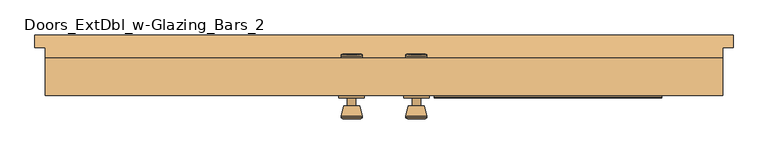
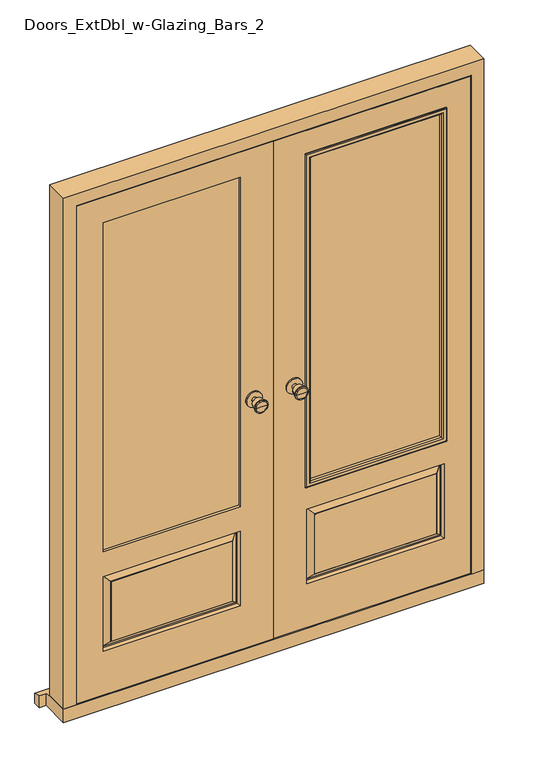
"""IFC4 building model written with IfcOpenShell, lengths in millimetres: door geometry, Doors_ExtDbl_w-Glazing_Bars_2."""

from ifc_helpers import new_model, si_unit, point, frame, frame_2d, origin, place, context, project, spatial, polyline, circle_curve, ellipse_curve, trimmed, segment, composite_curve, outline, extrude, faceted_brep, source, transform, mapped, element, save
from ifc_brep_helpers import plane_surface, cylinder_surface, revolved_surface, advanced_brep


def doors_extdbl_w_glazing_bars_2_f0b4ebcb(model_context):
    return source(origin(), model_context, "Body", "SolidModel", [
        advanced_brep(
        [(76.5, -5.7, 1050.0), (86.5, -5.7, 1050.0), (66.5, -5.7, 1050.0), (96.9758676, -54.7, 1050.0), (76.5, -54.7, 1050.0), (56.0241324, -54.7, 1050.0), (101.5, -52.8721319, 1050.0), (51.5, -52.8721319, 1050.0), (101.5, -49.4084537, 1050.0), (51.5, -49.4084537, 1050.0), (95.136236, -24.7, 1050.0), (57.863764, -24.7, 1050.0), (86.5, -24.7, 1050.0), (66.5, -24.7, 1050.0)],
        [
            (0, 1),
            (1, 2, circle_curve(frame((76.5, -5.7, 1050.0), z_axis=(0.0, 1.0, 0.0), x_axis=(-1.0, 0.0, 0.0)), 10.0)),
            (2, 0),
            (2, 1, circle_curve(frame((76.5, -5.7, 1050.0), z_axis=(0.0, 1.0, 0.0), x_axis=(-1.0, 0.0, 0.0)), 10.0)),
            (3, 4),
            (4, 5),
            (5, 3, circle_curve(frame((76.5, -54.7, 1050.0), z_axis=(0.0, -1.0, 0.0), x_axis=(-1.0, 0.0, 0.0)), 20.4758676)),
            (3, 5, circle_curve(frame((76.5, -54.7, 1050.0), z_axis=(0.0, -1.0, 0.0), x_axis=(-1.0, 0.0, 0.0)), 20.4758676)),
            (6, 3),
            (5, 7),
            (7, 6, circle_curve(frame((76.5, -52.8721319, 1050.0), z_axis=(0.0, -1.0, 0.0), x_axis=(-1.0, 0.0, 0.0)), 25.0)),
            (6, 7, circle_curve(frame((76.5, -52.8721319, 1050.0), z_axis=(0.0, -1.0, 0.0), x_axis=(-1.0, 0.0, 0.0)), 25.0)),
            (8, 6),
            (7, 9),
            (9, 8, circle_curve(frame((76.5, -49.4084537, 1050.0), z_axis=(0.0, -1.0, 0.0), x_axis=(-1.0, 0.0, 0.0)), 25.0)),
            (8, 9, circle_curve(frame((76.5, -49.4084537, 1050.0), z_axis=(0.0, -1.0, 0.0), x_axis=(-1.0, 0.0, 0.0)), 25.0)),
            (10, 8),
            (9, 11),
            (11, 10, circle_curve(frame((76.5, -24.7, 1050.0), z_axis=(0.0, -1.0, 0.0), x_axis=(-1.0, 0.0, 0.0)), 18.636236)),
            (10, 11, circle_curve(frame((76.5, -24.7, 1050.0), z_axis=(0.0, -1.0, 0.0), x_axis=(-1.0, 0.0, 0.0)), 18.636236)),
            (12, 10),
            (11, 13),
            (13, 12, circle_curve(frame((76.5, -24.7, 1050.0), z_axis=(0.0, -1.0, 0.0), x_axis=(-1.0, 0.0, 0.0)), 10.0)),
            (12, 13, circle_curve(frame((76.5, -24.7, 1050.0), z_axis=(0.0, -1.0, 0.0), x_axis=(-1.0, 0.0, 0.0)), 10.0)),
            (1, 12),
            (13, 2),
        ],
        [
            plane_surface(frame((76.5, -5.7, 1050.0), z_axis=(0.0, 1.0, 0.0), x_axis=(-1.0, 0.0, 0.0))),
            plane_surface(frame((76.5, -54.7, 1050.0), z_axis=(0.0, -1.0, 0.0), x_axis=(-1.0, 0.0, 0.0))),
            revolved_surface(polyline([(56.0241324, -54.7, 1050.0), (51.5, -52.8721319, 1050.0)]), (76.5, -5.7, 1050.0), (0.0, 1.0, 0.0)),
            cylinder_surface(frame((76.5, -5.7, 1050.0), z_axis=(0.0, 1.0, 0.0), x_axis=(-1.0, 0.0, 0.0)), 25.0),
            revolved_surface(polyline([(51.5, -49.4084537, 1050.0), (57.863764, -24.7, 1050.0)]), (76.5, -5.7, 1050.0), (0.0, 1.0, 0.0)),
            plane_surface(frame((76.5, -24.7, 1050.0), z_axis=(0.0, 1.0, 0.0), x_axis=(-1.0, 0.0, 0.0))),
            cylinder_surface(frame((76.5, -5.7, 1050.0), z_axis=(0.0, 1.0, 0.0), x_axis=(-1.0, 0.0, 0.0)), 10.0),
        ],
        [
            (0, [[1, 2, 3]]),
            (0, [[-3, 4, -1]]),
            (1, [[5, 6, 7]]),
            (1, [[-6, -5, 8]]),
            (2, [[9, -7, 10, 11]]),
            (2, [[-10, -8, -9, 12]]),
            (3, [[13, -11, 14, 15]]),
            (3, [[-14, -12, -13, 16]]),
            (4, [[17, -15, 18, 19]]),
            (4, [[-18, -16, -17, 20]]),
            (5, [[21, -19, 22, 23]]),
            (5, [[-22, -20, -21, 24]]),
            (6, [[25, -23, 26, -2]]),
            (6, [[-26, -24, -25, -4]]),
        ],
    ),
        extrude(outline(composite_curve([segment(trimmed(circle_curve(frame_2d((1050.0, 76.5)), 30.0), [point((1050.0, 46.5))], [point((1050.0, 106.5))], False, "CARTESIAN"), True, "CONTINUOUS"), segment(trimmed(circle_curve(frame_2d((1050.0, 76.5)), 30.0), [point((1050.0, 106.5))], [point((1050.0, 46.5))], False, "CARTESIAN"), True, "CONTINUOUS")], self_intersect=False)), frame((0.0, -5.7, 0.0), z_axis=(0.0, 1.0, 0.0), x_axis=(0.0, 0.0, 1.0)), (0.0, 0.0, 1.0), 6.0),
        advanced_brep(
        [(76.5, 50.3, 1050.0), (66.5, 50.3, 1050.0), (86.5, 50.3, 1050.0), (96.9758676, 99.3, 1050.0), (56.0241324, 99.3, 1050.0), (76.5, 99.3, 1050.0), (101.5, 97.4721319, 1050.0), (51.5, 97.4721319, 1050.0), (101.5, 94.0084537, 1050.0), (51.5, 94.0084537, 1050.0), (95.136236, 69.3, 1050.0), (57.863764, 69.3, 1050.0), (86.5, 69.3, 1050.0), (66.5, 69.3, 1050.0)],
        [
            (0, 1),
            (1, 2, circle_curve(frame((76.5, 50.3, 1050.0), z_axis=(0.0, -1.0, 0.0), x_axis=(-1.0, 0.0, 0.0)), 10.0)),
            (2, 0),
            (2, 1, circle_curve(frame((76.5, 50.3, 1050.0), z_axis=(0.0, -1.0, 0.0), x_axis=(-1.0, 0.0, 0.0)), 10.0)),
            (3, 4, circle_curve(frame((76.5, 99.3, 1050.0), z_axis=(0.0, 1.0, 0.0), x_axis=(-1.0, 0.0, 0.0)), 20.4758676)),
            (4, 5),
            (5, 3),
            (4, 3, circle_curve(frame((76.5, 99.3, 1050.0), z_axis=(0.0, 1.0, 0.0), x_axis=(-1.0, 0.0, 0.0)), 20.4758676)),
            (6, 7, circle_curve(frame((76.5, 97.4721319, 1050.0), z_axis=(0.0, 1.0, 0.0), x_axis=(-1.0, 0.0, 0.0)), 25.0)),
            (7, 4),
            (3, 6),
            (7, 6, circle_curve(frame((76.5, 97.4721319, 1050.0), z_axis=(0.0, 1.0, 0.0), x_axis=(-1.0, 0.0, 0.0)), 25.0)),
            (8, 9, circle_curve(frame((76.5, 94.0084537, 1050.0), z_axis=(0.0, 1.0, 0.0), x_axis=(-1.0, 0.0, 0.0)), 25.0)),
            (9, 7),
            (6, 8),
            (9, 8, circle_curve(frame((76.5, 94.0084537, 1050.0), z_axis=(0.0, 1.0, 0.0), x_axis=(-1.0, 0.0, 0.0)), 25.0)),
            (10, 11, circle_curve(frame((76.5, 69.3, 1050.0), z_axis=(0.0, 1.0, 0.0), x_axis=(-1.0, 0.0, 0.0)), 18.636236)),
            (11, 9),
            (8, 10),
            (11, 10, circle_curve(frame((76.5, 69.3, 1050.0), z_axis=(0.0, 1.0, 0.0), x_axis=(-1.0, 0.0, 0.0)), 18.636236)),
            (12, 13, circle_curve(frame((76.5, 69.3, 1050.0), z_axis=(0.0, 1.0, 0.0), x_axis=(-1.0, 0.0, 0.0)), 10.0)),
            (13, 11),
            (10, 12),
            (13, 12, circle_curve(frame((76.5, 69.3, 1050.0), z_axis=(0.0, 1.0, 0.0), x_axis=(-1.0, 0.0, 0.0)), 10.0)),
            (1, 13),
            (12, 2),
        ],
        [
            plane_surface(frame((76.5, 50.3, 1050.0), z_axis=(0.0, -1.0, 0.0), x_axis=(-1.0, 0.0, 0.0))),
            plane_surface(frame((76.5, 99.3, 1050.0), z_axis=(0.0, 1.0, 0.0), x_axis=(-1.0, 0.0, 0.0))),
            revolved_surface(polyline([(56.0241324, 99.3, 1050.0), (51.5, 97.4721319, 1050.0)]), (76.5, 50.3, 1050.0), (0.0, -1.0, 0.0)),
            cylinder_surface(frame((76.5, 50.3, 1050.0), z_axis=(0.0, -1.0, 0.0), x_axis=(-1.0, 0.0, 0.0)), 25.0),
            revolved_surface(polyline([(51.5, 94.0084537, 1050.0), (57.863764, 69.3, 1050.0)]), (76.5, 50.3, 1050.0), (0.0, -1.0, 0.0)),
            plane_surface(frame((76.5, 69.3, 1050.0), z_axis=(0.0, -1.0, 0.0), x_axis=(-1.0, 0.0, 0.0))),
            cylinder_surface(frame((76.5, 50.3, 1050.0), z_axis=(0.0, -1.0, 0.0), x_axis=(-1.0, 0.0, 0.0)), 10.0),
        ],
        [
            (0, [[1, 2, 3]]),
            (0, [[-3, 4, -1]]),
            (1, [[5, 6, 7]]),
            (1, [[8, -7, -6]]),
            (2, [[9, 10, -5, 11]]),
            (2, [[12, -11, -8, -10]]),
            (3, [[13, 14, -9, 15]]),
            (3, [[16, -15, -12, -14]]),
            (4, [[17, 18, -13, 19]]),
            (4, [[20, -19, -16, -18]]),
            (5, [[21, 22, -17, 23]]),
            (5, [[24, -23, -20, -22]]),
            (6, [[-2, 25, -21, 26]]),
            (6, [[-4, -26, -24, -25]]),
        ],
    ),
        extrude(outline(composite_curve([segment(trimmed(circle_curve(frame_2d((1050.0, 76.5)), 30.0), [point((1050.0, 46.5))], [point((1050.0, 106.5))], False, "CARTESIAN"), True, "CONTINUOUS"), segment(trimmed(circle_curve(frame_2d((1050.0, 76.5)), 30.0), [point((1050.0, 106.5))], [point((1050.0, 46.5))], False, "CARTESIAN"), True, "CONTINUOUS")], self_intersect=False)), frame((0.0, 44.3, 0.0), z_axis=(0.0, 1.0, 0.0), x_axis=(0.0, 0.0, 1.0)), (0.0, 0.0, 1.0), 6.0),
        advanced_brep(
        [(-76.5, -5.7, 1050.0), (-66.5, -5.7, 1050.0), (-86.5, -5.7, 1050.0), (-56.0241324, -54.7, 1050.0), (-76.5, -54.7, 1050.0), (-96.9758676, -54.7, 1050.0), (-51.5, -52.8721319, 1050.0), (-101.5, -52.8721319, 1050.0), (-51.5, -49.4084537, 1050.0), (-101.5, -49.4084537, 1050.0), (-57.863764, -24.7, 1050.0), (-95.136236, -24.7, 1050.0), (-66.5, -24.7, 1050.0), (-86.5, -24.7, 1050.0)],
        [
            (0, 1),
            (1, 2, circle_curve(frame((-76.5, -5.7, 1050.0), z_axis=(0.0, 1.0, 0.0), x_axis=(-1.0, 0.0, 0.0)), 10.0)),
            (2, 0),
            (2, 1, circle_curve(frame((-76.5, -5.7, 1050.0), z_axis=(0.0, 1.0, 0.0), x_axis=(-1.0, 0.0, 0.0)), 10.0)),
            (3, 4),
            (4, 5),
            (5, 3, circle_curve(frame((-76.5, -54.7, 1050.0), z_axis=(0.0, -1.0, 0.0), x_axis=(-1.0, 0.0, 0.0)), 20.4758676)),
            (3, 5, circle_curve(frame((-76.5, -54.7, 1050.0), z_axis=(0.0, -1.0, 0.0), x_axis=(-1.0, 0.0, 0.0)), 20.4758676)),
            (6, 3),
            (5, 7),
            (7, 6, circle_curve(frame((-76.5, -52.8721319, 1050.0), z_axis=(0.0, -1.0, 0.0), x_axis=(-1.0, 0.0, 0.0)), 25.0)),
            (6, 7, circle_curve(frame((-76.5, -52.8721319, 1050.0), z_axis=(0.0, -1.0, 0.0), x_axis=(-1.0, 0.0, 0.0)), 25.0)),
            (8, 6),
            (7, 9),
            (9, 8, circle_curve(frame((-76.5, -49.4084537, 1050.0), z_axis=(0.0, -1.0, 0.0), x_axis=(-1.0, 0.0, 0.0)), 25.0)),
            (8, 9, circle_curve(frame((-76.5, -49.4084537, 1050.0), z_axis=(0.0, -1.0, 0.0), x_axis=(-1.0, 0.0, 0.0)), 25.0)),
            (10, 8),
            (9, 11),
            (11, 10, circle_curve(frame((-76.5, -24.7, 1050.0), z_axis=(0.0, -1.0, 0.0), x_axis=(-1.0, 0.0, 0.0)), 18.636236)),
            (10, 11, circle_curve(frame((-76.5, -24.7, 1050.0), z_axis=(0.0, -1.0, 0.0), x_axis=(-1.0, 0.0, 0.0)), 18.636236)),
            (12, 10),
            (11, 13),
            (13, 12, circle_curve(frame((-76.5, -24.7, 1050.0), z_axis=(0.0, -1.0, 0.0), x_axis=(-1.0, 0.0, 0.0)), 10.0)),
            (12, 13, circle_curve(frame((-76.5, -24.7, 1050.0), z_axis=(0.0, -1.0, 0.0), x_axis=(-1.0, 0.0, 0.0)), 10.0)),
            (1, 12),
            (13, 2),
        ],
        [
            plane_surface(frame((-76.5, -5.7, 1050.0), z_axis=(0.0, 1.0, 0.0), x_axis=(-1.0, 0.0, 0.0))),
            plane_surface(frame((-76.5, -54.7, 1050.0), z_axis=(0.0, -1.0, 0.0), x_axis=(-1.0, 0.0, 0.0))),
            revolved_surface(polyline([(-96.9758676, -54.7, 1050.0), (-101.5, -52.8721319, 1050.0)]), (-76.5, -5.7, 1050.0), (0.0, 1.0, 0.0)),
            cylinder_surface(frame((-76.5, -5.7, 1050.0), z_axis=(0.0, 1.0, 0.0), x_axis=(-1.0, 0.0, 0.0)), 25.0),
            revolved_surface(polyline([(-101.5, -49.4084537, 1050.0), (-95.136236, -24.7, 1050.0)]), (-76.5, -5.7, 1050.0), (0.0, 1.0, 0.0)),
            plane_surface(frame((-76.5, -24.7, 1050.0), z_axis=(0.0, 1.0, 0.0), x_axis=(-1.0, 0.0, 0.0))),
            cylinder_surface(frame((-76.5, -5.7, 1050.0), z_axis=(0.0, 1.0, 0.0), x_axis=(-1.0, 0.0, 0.0)), 10.0),
        ],
        [
            (0, [[1, 2, 3]]),
            (0, [[-3, 4, -1]]),
            (1, [[5, 6, 7]]),
            (1, [[-6, -5, 8]]),
            (2, [[9, -7, 10, 11]]),
            (2, [[-10, -8, -9, 12]]),
            (3, [[13, -11, 14, 15]]),
            (3, [[-14, -12, -13, 16]]),
            (4, [[17, -15, 18, 19]]),
            (4, [[-18, -16, -17, 20]]),
            (5, [[21, -19, 22, 23]]),
            (5, [[-22, -20, -21, 24]]),
            (6, [[25, -23, 26, -2]]),
            (6, [[-26, -24, -25, -4]]),
        ],
    ),
        extrude(outline(composite_curve([segment(trimmed(circle_curve(frame_2d((1050.0, -76.5)), 30.0), [point((1050.0, -106.5))], [point((1050.0, -46.5))], False, "CARTESIAN"), True, "CONTINUOUS"), segment(trimmed(circle_curve(frame_2d((1050.0, -76.5)), 30.0), [point((1050.0, -46.5))], [point((1050.0, -106.5))], False, "CARTESIAN"), True, "CONTINUOUS")], self_intersect=False)), frame((0.0, -5.7, 0.0), z_axis=(0.0, 1.0, 0.0), x_axis=(0.0, 0.0, 1.0)), (0.0, 0.0, 1.0), 6.0),
        advanced_brep(
        [(-76.5, 50.3, 1050.0), (-86.5, 50.3, 1050.0), (-66.5, 50.3, 1050.0), (-56.0241324, 99.3, 1050.0), (-96.9758676, 99.3, 1050.0), (-76.5, 99.3, 1050.0), (-51.5, 97.4721319, 1050.0), (-101.5, 97.4721319, 1050.0), (-51.5, 94.0084537, 1050.0), (-101.5, 94.0084537, 1050.0), (-57.863764, 69.3, 1050.0), (-95.136236, 69.3, 1050.0), (-66.5, 69.3, 1050.0), (-86.5, 69.3, 1050.0)],
        [
            (0, 1),
            (1, 2, circle_curve(frame((-76.5, 50.3, 1050.0), z_axis=(0.0, -1.0, 0.0), x_axis=(-1.0, 0.0, 0.0)), 10.0)),
            (2, 0),
            (2, 1, circle_curve(frame((-76.5, 50.3, 1050.0), z_axis=(0.0, -1.0, 0.0), x_axis=(-1.0, 0.0, 0.0)), 10.0)),
            (3, 4, circle_curve(frame((-76.5, 99.3, 1050.0), z_axis=(0.0, 1.0, 0.0), x_axis=(-1.0, 0.0, 0.0)), 20.4758676)),
            (4, 5),
            (5, 3),
            (4, 3, circle_curve(frame((-76.5, 99.3, 1050.0), z_axis=(0.0, 1.0, 0.0), x_axis=(-1.0, 0.0, 0.0)), 20.4758676)),
            (6, 7, circle_curve(frame((-76.5, 97.4721319, 1050.0), z_axis=(0.0, 1.0, 0.0), x_axis=(-1.0, 0.0, 0.0)), 25.0)),
            (7, 4),
            (3, 6),
            (7, 6, circle_curve(frame((-76.5, 97.4721319, 1050.0), z_axis=(0.0, 1.0, 0.0), x_axis=(-1.0, 0.0, 0.0)), 25.0)),
            (8, 9, circle_curve(frame((-76.5, 94.0084537, 1050.0), z_axis=(0.0, 1.0, 0.0), x_axis=(-1.0, 0.0, 0.0)), 25.0)),
            (9, 7),
            (6, 8),
            (9, 8, circle_curve(frame((-76.5, 94.0084537, 1050.0), z_axis=(0.0, 1.0, 0.0), x_axis=(-1.0, 0.0, 0.0)), 25.0)),
            (10, 11, circle_curve(frame((-76.5, 69.3, 1050.0), z_axis=(0.0, 1.0, 0.0), x_axis=(-1.0, 0.0, 0.0)), 18.636236)),
            (11, 9),
            (8, 10),
            (11, 10, circle_curve(frame((-76.5, 69.3, 1050.0), z_axis=(0.0, 1.0, 0.0), x_axis=(-1.0, 0.0, 0.0)), 18.636236)),
            (12, 13, circle_curve(frame((-76.5, 69.3, 1050.0), z_axis=(0.0, 1.0, 0.0), x_axis=(-1.0, 0.0, 0.0)), 10.0)),
            (13, 11),
            (10, 12),
            (13, 12, circle_curve(frame((-76.5, 69.3, 1050.0), z_axis=(0.0, 1.0, 0.0), x_axis=(-1.0, 0.0, 0.0)), 10.0)),
            (1, 13),
            (12, 2),
        ],
        [
            plane_surface(frame((-76.5, 50.3, 1050.0), z_axis=(0.0, -1.0, 0.0), x_axis=(-1.0, 0.0, 0.0))),
            plane_surface(frame((-76.5, 99.3, 1050.0), z_axis=(0.0, 1.0, 0.0), x_axis=(-1.0, 0.0, 0.0))),
            revolved_surface(polyline([(-96.9758676, 99.3, 1050.0), (-101.5, 97.4721319, 1050.0)]), (-76.5, 50.3, 1050.0), (0.0, -1.0, 0.0)),
            cylinder_surface(frame((-76.5, 50.3, 1050.0), z_axis=(0.0, -1.0, 0.0), x_axis=(-1.0, 0.0, 0.0)), 25.0),
            revolved_surface(polyline([(-101.5, 94.0084537, 1050.0), (-95.136236, 69.3, 1050.0)]), (-76.5, 50.3, 1050.0), (0.0, -1.0, 0.0)),
            plane_surface(frame((-76.5, 69.3, 1050.0), z_axis=(0.0, -1.0, 0.0), x_axis=(-1.0, 0.0, 0.0))),
            cylinder_surface(frame((-76.5, 50.3, 1050.0), z_axis=(0.0, -1.0, 0.0), x_axis=(-1.0, 0.0, 0.0)), 10.0),
        ],
        [
            (0, [[1, 2, 3]]),
            (0, [[-3, 4, -1]]),
            (1, [[5, 6, 7]]),
            (1, [[8, -7, -6]]),
            (2, [[9, 10, -5, 11]]),
            (2, [[12, -11, -8, -10]]),
            (3, [[13, 14, -9, 15]]),
            (3, [[16, -15, -12, -14]]),
            (4, [[17, 18, -13, 19]]),
            (4, [[20, -19, -16, -18]]),
            (5, [[21, 22, -17, 23]]),
            (5, [[24, -23, -20, -22]]),
            (6, [[-2, 25, -21, 26]]),
            (6, [[-4, -26, -24, -25]]),
        ],
    ),
        extrude(outline(composite_curve([segment(trimmed(circle_curve(frame_2d((1050.0, -76.5)), 30.0), [point((1050.0, -106.5))], [point((1050.0, -46.5))], False, "CARTESIAN"), True, "CONTINUOUS"), segment(trimmed(circle_curve(frame_2d((1050.0, -76.5)), 30.0), [point((1050.0, -46.5))], [point((1050.0, -106.5))], False, "CARTESIAN"), True, "CONTINUOUS")], self_intersect=False)), frame((0.0, 44.3, 0.0), z_axis=(0.0, 1.0, 0.0), x_axis=(0.0, 0.0, 1.0)), (0.0, 0.0, 1.0), 6.0),
        faceted_brep([(729.5, 89.3, 54.5), (800.0, 89.3, 54.5), (800.0, 0.3, 54.5), (751.5, 0.3, 54.5), (751.5, 47.3, 54.5), (729.5, 47.3, 54.5), (729.5, 89.3, 2039.5), (-729.5, 89.3, 2039.5), (-729.5, 89.3, 54.5), (-800.0, 89.3, 54.5), (-800.0, 89.3, 2110.0), (800.0, 89.3, 2110.0), (800.0, 0.3, 2110.0), (-800.0, 0.3, 2110.0), (-800.0, 0.3, 54.5), (-751.5, 0.3, 54.5), (-751.5, 0.3, 2061.5), (751.5, 0.3, 2061.5), (751.5, 47.3, 2061.5), (-751.5, 47.3, 2061.5), (-751.5, 47.3, 54.5), (-729.5, 47.3, 54.5), (-729.5, 47.3, 2039.5), (729.5, 47.3, 2039.5)], [[[0, 1, 2, 3, 4, 5]], [[1, 0, 6, 7, 8, 9, 10, 11]], [[2, 1, 11, 12]], [[3, 2, 12, 13, 14, 15, 16, 17]], [[4, 3, 17, 18]], [[5, 4, 18, 19, 20, 21, 22, 23]], [[0, 5, 23, 6]], [[8, 7, 22, 21]], [[9, 8, 21, 20, 15, 14]], [[10, 9, 14, 13]], [[16, 15, 20, 19]], [[11, 10, 13, 12]], [[17, 16, 19, 18]], [[7, 6, 23, 22]]]),
        faceted_brep([(748.5, 0.3, 58.5), (748.5, 0.3, 2058.5), (1.5, 0.3, 2058.5), (1.5, 0.3, 58.5), (648.5, 0.3, 1958.5), (648.5, 0.3, 633.5), (126.5, 0.3, 633.5), (126.5, 0.3, 1958.5), (648.5, 0.3, 533.5), (648.5, 0.3, 233.5), (126.5, 0.3, 233.5), (126.5, 0.3, 533.5), (618.5, 0.3, 263.5), (618.5, 0.3, 503.5), (156.5, 0.3, 503.5), (156.5, 0.3, 263.5), (748.5, 44.3, 58.5), (1.5, 44.3, 58.5), (1.5, 44.3, 2058.5), (748.5, 44.3, 2058.5), (648.5, 44.3, 1958.5), (126.5, 44.3, 1958.5), (126.5, 44.3, 633.5), (648.5, 44.3, 633.5), (126.5, 44.3, 533.5), (126.5, 44.3, 233.5), (648.5, 44.3, 233.5), (648.5, 44.3, 533.5), (156.5, 44.3, 263.5), (156.5, 44.3, 503.5), (618.5, 44.3, 503.5), (618.5, 44.3, 263.5), (129.5, 29.3, 530.5), (129.5, 29.3, 236.5), (154.5, 43.3, 505.5), (154.5, 43.3, 261.5), (134.5, 29.3, 241.5), (134.5, 29.3, 525.5), (156.5, 43.3, 263.5), (156.5, 43.3, 503.5), (645.5, 29.3, 236.5), (620.5, 43.3, 261.5), (640.5, 29.3, 241.5), (618.5, 43.3, 263.5), (645.5, 29.3, 530.5), (620.5, 43.3, 505.5), (640.5, 29.3, 525.5), (618.5, 43.3, 503.5), (645.5, 15.3, 530.5), (645.5, 15.3, 236.5), (620.5, 1.3, 505.5), (620.5, 1.3, 261.5), (640.5, 15.3, 241.5), (640.5, 15.3, 525.5), (618.5, 1.3, 263.5), (618.5, 1.3, 503.5), (129.5, 15.3, 236.5), (154.5, 1.3, 261.5), (134.5, 15.3, 241.5), (156.5, 1.3, 263.5), (129.5, 15.3, 530.5), (154.5, 1.3, 505.5), (134.5, 15.3, 525.5), (156.5, 1.3, 503.5)], [[[0, 1, 2, 3], [4, 5, 6, 7], [8, 9, 10, 11]], [[12, 13, 14, 15]], [[16, 17, 18, 19], [20, 21, 22, 23], [24, 25, 26, 27]], [[28, 29, 30, 31]], [[1, 0, 16, 19]], [[2, 1, 19, 18]], [[3, 2, 18, 17]], [[0, 3, 17, 16]], [[5, 4, 20, 23]], [[6, 5, 23, 22]], [[7, 6, 22, 21]], [[4, 7, 21, 20]], [[32, 33, 25, 24]], [[34, 35, 36, 37]], [[28, 38, 39, 29]], [[25, 33, 40, 26]], [[36, 35, 41, 42]], [[38, 28, 31, 43]], [[26, 40, 44, 27]], [[42, 41, 45, 46]], [[43, 31, 30, 47]], [[32, 24, 27, 44]], [[33, 32, 44, 40], [37, 36, 42, 46]], [[34, 37, 46, 45]], [[35, 34, 45, 41], [39, 38, 43, 47]], [[29, 39, 47, 30]], [[48, 49, 9, 8]], [[50, 51, 52, 53]], [[12, 54, 55, 13]], [[9, 49, 56, 10]], [[52, 51, 57, 58]], [[54, 12, 15, 59]], [[10, 56, 60, 11]], [[58, 57, 61, 62]], [[59, 15, 14, 63]], [[48, 8, 11, 60]], [[49, 48, 60, 56], [53, 52, 58, 62]], [[50, 53, 62, 61]], [[51, 50, 61, 57], [55, 54, 59, 63]], [[13, 55, 63, 14]]]),
        faceted_brep([(-748.5, 0.3, 58.5), (-1.5, 0.3, 58.5), (-1.5, 0.3, 2058.5), (-748.5, 0.3, 2058.5), (-126.5, 0.3, 1958.5), (-126.5, 0.3, 633.5), (-648.5, 0.3, 633.5), (-648.5, 0.3, 1958.5), (-126.5, 0.3, 533.5), (-126.5, 0.3, 233.5), (-648.5, 0.3, 233.5), (-648.5, 0.3, 533.5), (-156.5, 0.3, 263.5), (-156.5, 0.3, 503.5), (-618.5, 0.3, 503.5), (-618.5, 0.3, 263.5), (-748.5, 44.3, 58.5), (-748.5, 44.3, 2058.5), (-1.5, 44.3, 2058.5), (-1.5, 44.3, 58.5), (-126.5, 44.3, 1958.5), (-648.5, 44.3, 1958.5), (-648.5, 44.3, 633.5), (-126.5, 44.3, 633.5), (-648.5, 44.3, 533.5), (-648.5, 44.3, 233.5), (-126.5, 44.3, 233.5), (-126.5, 44.3, 533.5), (-618.5, 44.3, 263.5), (-618.5, 44.3, 503.5), (-156.5, 44.3, 503.5), (-156.5, 44.3, 263.5), (-618.5, 43.3, 263.5), (-618.5, 43.3, 503.5), (-640.5, 29.3, 241.5), (-640.5, 29.3, 525.5), (-620.5, 43.3, 505.5), (-620.5, 43.3, 261.5), (-645.5, 29.3, 530.5), (-645.5, 29.3, 236.5), (-156.5, 43.3, 503.5), (-134.5, 29.3, 525.5), (-154.5, 43.3, 505.5), (-129.5, 29.3, 530.5), (-156.5, 43.3, 263.5), (-134.5, 29.3, 241.5), (-154.5, 43.3, 261.5), (-129.5, 29.3, 236.5), (-129.5, 15.3, 530.5), (-129.5, 15.3, 236.5), (-154.5, 1.3, 505.5), (-154.5, 1.3, 261.5), (-134.5, 15.3, 241.5), (-134.5, 15.3, 525.5), (-156.5, 1.3, 263.5), (-156.5, 1.3, 503.5), (-645.5, 15.3, 236.5), (-620.5, 1.3, 261.5), (-640.5, 15.3, 241.5), (-618.5, 1.3, 263.5), (-645.5, 15.3, 530.5), (-620.5, 1.3, 505.5), (-640.5, 15.3, 525.5), (-618.5, 1.3, 503.5)], [[[0, 1, 2, 3], [4, 5, 6, 7], [8, 9, 10, 11]], [[12, 13, 14, 15]], [[16, 17, 18, 19], [20, 21, 22, 23], [24, 25, 26, 27]], [[28, 29, 30, 31]], [[1, 0, 16, 19]], [[2, 1, 19, 18]], [[3, 2, 18, 17]], [[0, 3, 17, 16]], [[5, 4, 20, 23]], [[6, 5, 23, 22]], [[7, 6, 22, 21]], [[4, 7, 21, 20]], [[32, 33, 29, 28]], [[34, 35, 36, 37]], [[24, 38, 39, 25]], [[29, 33, 40, 30]], [[36, 35, 41, 42]], [[38, 24, 27, 43]], [[30, 40, 44, 31]], [[42, 41, 45, 46]], [[43, 27, 26, 47]], [[32, 28, 31, 44]], [[37, 36, 42, 46], [33, 32, 44, 40]], [[34, 37, 46, 45]], [[39, 38, 43, 47], [35, 34, 45, 41]], [[25, 39, 47, 26]], [[48, 49, 9, 8]], [[50, 51, 52, 53]], [[12, 54, 55, 13]], [[9, 49, 56, 10]], [[52, 51, 57, 58]], [[54, 12, 15, 59]], [[10, 56, 60, 11]], [[58, 57, 61, 62]], [[59, 15, 14, 63]], [[48, 8, 11, 60]], [[49, 48, 60, 56], [53, 52, 58, 62]], [[50, 53, 62, 61]], [[51, 50, 61, 57], [55, 54, 59, 63]], [[13, 55, 63, 14]]]),
        faceted_brep([(825.0, 144.3, 0.0), (825.0, 144.3, 38.5947221), (825.0, 114.3, 47.2703282), (825.0, 114.3, 0.0), (-825.0, 144.3, 38.5947221), (-825.0, 144.3, 0.0), (-825.0, 114.3, 0.0), (-825.0, 114.3, 47.2703282), (800.0, 114.3, 0.0), (800.0, 0.3, 0.0), (-800.0, 0.3, 0.0), (-800.0, 114.3, 0.0), (-800.0, 114.3, 47.2703282), (-800.0, 89.3, 54.5), (800.0, 89.3, 54.5), (800.0, 114.3, 47.2703282), (-800.0, 0.3, 54.5), (800.0, 0.3, 54.5)], [[[0, 1, 2, 3]], [[4, 5, 6, 7]], [[5, 0, 3, 8, 9, 10, 11, 6]], [[1, 0, 5, 4]], [[1, 4, 7, 12, 13, 14, 15, 2]], [[13, 16, 17, 14]], [[16, 10, 9, 17]], [[12, 11, 10, 16, 13]], [[11, 12, 7, 6]], [[8, 15, 14, 17, 9]], [[15, 8, 3, 2]]]),
        extrude(outline(polyline([(126.5, 34.3), (648.5, 34.3), (648.5, 10.3), (126.5, 10.3), (126.5, 34.3)])), frame((0.0, 0.0, 633.5), z_axis=(0.0, 0.0, 1.0), x_axis=(1.0, 0.0, 0.0)), (0.0, 0.0, 1.0), 1325.0),
        extrude(outline(polyline([(-648.5, 34.3), (-126.5, 34.3), (-126.5, 10.3), (-648.5, 10.3), (-648.5, 34.3)])), frame((0.0, 0.0, 633.5), z_axis=(0.0, 0.0, 1.0), x_axis=(1.0, 0.0, 0.0)), (0.0, 0.0, 1.0), 1325.0),
        advanced_brep(
        [(118.5, 48.3, 625.5), (118.5, 44.3, 625.5), (118.5, 44.3, 1966.5), (118.5, 48.3, 1966.5), (120.5, 50.3, 627.5), (120.5, 50.3, 1964.5), (138.5, 45.3, 645.5), (133.5, 50.3, 640.5), (133.5, 50.3, 1951.5), (138.5, 45.3, 1946.5), (138.5, 34.3, 645.5), (138.5, 34.3, 1946.5), (126.5, 44.3, 633.5), (126.5, 34.3, 633.5), (126.5, 34.3, 1958.5), (126.5, 44.3, 1958.5), (656.5, 44.3, 1966.5), (656.5, 48.3, 1966.5), (654.5, 50.3, 1964.5), (641.5, 50.3, 1951.5), (636.5, 45.3, 1946.5), (636.5, 34.3, 1946.5), (648.5, 34.3, 1958.5), (648.5, 44.3, 1958.5), (656.5, 44.3, 625.5), (656.5, 48.3, 625.5), (654.5, 50.3, 627.5), (641.5, 50.3, 640.5), (636.5, 45.3, 645.5), (636.5, 34.3, 645.5), (648.5, 34.3, 633.5), (648.5, 44.3, 633.5)],
        [
            (0, 1),
            (1, 2),
            (2, 3),
            (3, 0),
            (4, 0, ellipse_curve(frame((120.5, 48.3, 627.5), z_axis=(-0.7071067811865476, 0.0, 0.7071067811865475), x_axis=(-0.7071067811865475, 0.0, -0.7071067811865476)), 2.8284271, 2.0)),
            (3, 5, ellipse_curve(frame((120.5, 48.3, 1964.5), z_axis=(-0.7071067811865475, 0.0, -0.7071067811865476), x_axis=(0.7071067811865476, 0.0, -0.7071067811865475)), 2.8284271, 2.0)),
            (5, 4),
            (6, 7, ellipse_curve(frame((133.5, 45.3, 640.5), z_axis=(-0.7071067811865476, 0.0, 0.7071067811865475), x_axis=(-0.7071067811865475, 0.0, -0.7071067811865476)), 7.0710678, 5.0)),
            (7, 8),
            (8, 9, ellipse_curve(frame((133.5, 45.3, 1951.5), z_axis=(-0.7071067811865475, 0.0, -0.7071067811865476), x_axis=(0.7071067811865476, 0.0, -0.7071067811865475)), 7.0710678, 5.0)),
            (9, 6),
            (10, 6),
            (9, 11),
            (11, 10),
            (12, 13),
            (13, 14),
            (14, 15),
            (15, 12),
            (2, 16),
            (16, 17),
            (17, 3),
            (17, 18, ellipse_curve(frame((654.5, 48.3, 1964.5), z_axis=(-0.7071067811865476, 0.0, 0.7071067811865475), x_axis=(-0.7071067811865475, 0.0, -0.7071067811865476)), 2.8284271, 2.0)),
            (18, 5),
            (8, 19),
            (19, 20, ellipse_curve(frame((641.5, 45.3, 1951.5), z_axis=(-0.7071067811865476, 0.0, 0.7071067811865475), x_axis=(-0.7071067811865475, 0.0, -0.7071067811865476)), 7.0710678, 5.0)),
            (20, 9),
            (20, 21),
            (21, 11),
            (14, 22),
            (22, 23),
            (23, 15),
            (16, 24),
            (24, 25),
            (25, 17),
            (25, 26, ellipse_curve(frame((654.5, 48.3, 627.5), z_axis=(0.7071067811865475, 0.0, 0.7071067811865476), x_axis=(-0.7071067811865476, 0.0, 0.7071067811865475)), 2.8284271, 2.0)),
            (26, 18),
            (19, 27),
            (27, 28, ellipse_curve(frame((641.5, 45.3, 640.5), z_axis=(0.7071067811865475, 0.0, 0.7071067811865476), x_axis=(-0.7071067811865476, 0.0, 0.7071067811865475)), 7.0710678, 5.0)),
            (28, 20),
            (28, 29),
            (29, 21),
            (22, 30),
            (30, 31),
            (31, 23),
            (24, 1),
            (0, 25),
            (4, 26),
            (7, 27),
            (6, 28),
            (10, 29),
            (13, 30),
            (12, 31),
        ],
        [
            plane_surface(frame((118.5, 44.3, 625.5), z_axis=(-1.0, 0.0, 0.0), x_axis=(0.0, 0.0, 1.0))),
            cylinder_surface(frame((120.5, 48.3, 633.5), z_axis=(0.0, 0.0, -1.0), x_axis=(-1.0, 0.0, 0.0)), 2.0),
            cylinder_surface(frame((133.5, 45.3, 633.5), z_axis=(0.0, 0.0, -1.0), x_axis=(-1.0, 0.0, 0.0)), 5.0),
            plane_surface(frame((138.5, 45.3, 645.5), z_axis=(1.0, 0.0, 0.0), x_axis=(0.0, 0.0, 1.0))),
            plane_surface(frame((126.5, 34.3, 633.5), z_axis=(-1.0, 0.0, 0.0), x_axis=(0.0, 0.0, 1.0))),
            plane_surface(frame((118.5, 44.3, 1966.5), z_axis=(0.0, 0.0, 1.0), x_axis=(1.0, 0.0, 0.0))),
            cylinder_surface(frame((126.5, 48.3, 1964.5), z_axis=(-1.0, 0.0, 0.0), x_axis=(0.0, 0.0, 1.0)), 2.0),
            cylinder_surface(frame((126.5, 45.3, 1951.5), z_axis=(-1.0, 0.0, 0.0), x_axis=(0.0, 0.0, 1.0)), 5.0),
            plane_surface(frame((138.5, 45.3, 1946.5), z_axis=(0.0, 0.0, -1.0), x_axis=(1.0, 0.0, 0.0))),
            plane_surface(frame((126.5, 34.3, 1958.5), z_axis=(0.0, 0.0, 1.0), x_axis=(1.0, 0.0, 0.0))),
            plane_surface(frame((656.5, 44.3, 1966.5), z_axis=(1.0, 0.0, 0.0), x_axis=(0.0, 0.0, -1.0))),
            cylinder_surface(frame((654.5, 48.3, 1958.5), z_axis=(0.0, 0.0, 1.0), x_axis=(1.0, 0.0, 0.0)), 2.0),
            cylinder_surface(frame((641.5, 45.3, 1958.5), z_axis=(0.0, 0.0, 1.0), x_axis=(1.0, 0.0, 0.0)), 5.0),
            plane_surface(frame((636.5, 45.3, 1946.5), z_axis=(-1.0, 0.0, 0.0), x_axis=(0.0, 0.0, -1.0))),
            plane_surface(frame((648.5, 34.3, 1958.5), z_axis=(1.0, 0.0, 0.0), x_axis=(0.0, 0.0, -1.0))),
            plane_surface(frame((656.5, 44.3, 625.5), z_axis=(0.0, 0.0, -1.0), x_axis=(-1.0, 0.0, 0.0))),
            cylinder_surface(frame((648.5, 48.3, 627.5), z_axis=(1.0, 0.0, 0.0), x_axis=(0.0, 0.0, -1.0)), 2.0),
            plane_surface(frame((654.5, 50.3, 627.5), z_axis=(0.0, 1.0, 0.0), x_axis=(-1.0, 0.0, 0.0))),
            cylinder_surface(frame((648.5, 45.3, 640.5), z_axis=(1.0, 0.0, 0.0), x_axis=(0.0, 0.0, -1.0)), 5.0),
            plane_surface(frame((636.5, 45.3, 645.5), z_axis=(0.0, 0.0, 1.0), x_axis=(-1.0, 0.0, 0.0))),
            plane_surface(frame((636.5, 34.3, 645.5), z_axis=(0.0, -1.0, 0.0), x_axis=(-1.0, 0.0, 0.0))),
            plane_surface(frame((648.5, 34.3, 633.5), z_axis=(0.0, 0.0, -1.0), x_axis=(-1.0, 0.0, 0.0))),
            plane_surface(frame((648.5, 44.3, 633.5), z_axis=(0.0, -1.0, 0.0), x_axis=(-1.0, 0.0, 0.0))),
        ],
        [
            (0, [[1, 2, 3, 4]]),
            (1, [[5, -4, 6, 7]]),
            (2, [[8, 9, 10, 11]]),
            (3, [[12, -11, 13, 14]]),
            (4, [[15, 16, 17, 18]]),
            (5, [[-3, 19, 20, 21]]),
            (6, [[-6, -21, 22, 23]]),
            (7, [[-10, 24, 25, 26]]),
            (8, [[-13, -26, 27, 28]]),
            (9, [[-17, 29, 30, 31]]),
            (10, [[-20, 32, 33, 34]]),
            (11, [[-22, -34, 35, 36]]),
            (12, [[-25, 37, 38, 39]]),
            (13, [[-27, -39, 40, 41]]),
            (14, [[-30, 42, 43, 44]]),
            (15, [[-33, 45, -1, 46]]),
            (16, [[-35, -46, -5, 47]]),
            (17, [[-23, -36, -47, -7], [48, -37, -24, -9]]),
            (18, [[-38, -48, -8, 49]]),
            (19, [[-40, -49, -12, 50]]),
            (20, [[51, -42, -29, -16], [-28, -41, -50, -14]]),
            (21, [[-43, -51, -15, 52]]),
            (22, [[-45, -32, -19, -2], [-31, -44, -52, -18]]),
        ],
    ),
        advanced_brep(
        [(648.5, 10.3, 1958.5), (648.5, 0.3, 1958.5), (648.5, 0.3, 633.5), (648.5, 10.3, 633.5), (636.5, -0.7, 1946.5), (636.5, 10.3, 1946.5), (636.5, 10.3, 645.5), (636.5, -0.7, 645.5), (641.5, -5.7, 1951.5), (641.5, -5.7, 640.5), (656.5, -3.7, 1966.5), (654.5, -5.7, 1964.5), (654.5, -5.7, 627.5), (656.5, -3.7, 625.5), (656.5, 0.3, 1966.5), (656.5, 0.3, 625.5), (126.5, 0.3, 633.5), (126.5, 10.3, 633.5), (138.5, 10.3, 645.5), (138.5, -0.7, 645.5), (133.5, -5.7, 640.5), (120.5, -5.7, 627.5), (118.5, -3.7, 625.5), (118.5, 0.3, 625.5), (126.5, 0.3, 1958.5), (126.5, 10.3, 1958.5), (138.5, 10.3, 1946.5), (138.5, -0.7, 1946.5), (133.5, -5.7, 1951.5), (120.5, -5.7, 1964.5), (118.5, -3.7, 1966.5), (118.5, 0.3, 1966.5)],
        [
            (0, 1),
            (1, 2),
            (2, 3),
            (3, 0),
            (4, 5),
            (5, 6),
            (6, 7),
            (7, 4),
            (8, 4, ellipse_curve(frame((641.5, -0.7, 1951.5), z_axis=(0.7071067811865519, 0.0, -0.707106781186543), x_axis=(0.707106781186543, 0.0, 0.7071067811865521)), 7.0710678, 5.0)),
            (7, 9, ellipse_curve(frame((641.5, -0.7, 640.5), z_axis=(0.7071067811865429, 0.0, 0.707106781186552), x_axis=(-0.7071067811865519, 0.0, 0.707106781186543)), 7.0710678, 5.0)),
            (9, 8),
            (10, 11, ellipse_curve(frame((654.5, -3.7, 1964.5), z_axis=(0.7071067811865519, 0.0, -0.707106781186543), x_axis=(0.707106781186543, 0.0, 0.7071067811865521)), 2.8284271, 2.0)),
            (11, 12),
            (12, 13, ellipse_curve(frame((654.5, -3.7, 627.5), z_axis=(0.7071067811865429, 0.0, 0.707106781186552), x_axis=(-0.7071067811865519, 0.0, 0.707106781186543)), 2.8284271, 2.0)),
            (13, 10),
            (14, 10),
            (13, 15),
            (15, 14),
            (2, 16),
            (16, 17),
            (17, 3),
            (6, 18),
            (18, 19),
            (19, 7),
            (19, 20, ellipse_curve(frame((133.5, -0.7, 640.5), z_axis=(0.707106781186552, 0.0, -0.7071067811865429), x_axis=(0.707106781186543, 0.0, 0.7071067811865519)), 7.0710678, 5.0)),
            (20, 9),
            (12, 21),
            (21, 22, ellipse_curve(frame((120.5, -3.7, 627.5), z_axis=(0.707106781186552, 0.0, -0.7071067811865429), x_axis=(0.707106781186543, 0.0, 0.7071067811865519)), 2.8284271, 2.0)),
            (22, 13),
            (22, 23),
            (23, 15),
            (16, 24),
            (24, 25),
            (25, 17),
            (18, 26),
            (26, 27),
            (27, 19),
            (27, 28, ellipse_curve(frame((133.5, -0.7, 1951.5), z_axis=(-0.7071067811865431, 0.0, -0.707106781186552), x_axis=(0.7071067811865521, 0.0, -0.7071067811865429)), 7.0710678, 5.0)),
            (28, 20),
            (21, 29),
            (29, 30, ellipse_curve(frame((120.5, -3.7, 1964.5), z_axis=(-0.7071067811865431, 0.0, -0.707106781186552), x_axis=(0.7071067811865521, 0.0, -0.7071067811865429)), 2.8284271, 2.0)),
            (30, 22),
            (30, 31),
            (31, 23),
            (31, 14),
            (1, 24),
            (0, 25),
            (5, 26),
            (4, 27),
            (8, 28),
            (11, 29),
            (10, 30),
        ],
        [
            plane_surface(frame((648.5, 0.3, 1958.5), z_axis=(1.0, 0.0, 0.0), x_axis=(0.0, 0.0, -1.0))),
            plane_surface(frame((636.5, 10.3, 1946.5), z_axis=(-1.0, 0.0, 0.0), x_axis=(0.0, 0.0, -1.0))),
            cylinder_surface(frame((641.5, -0.7, 1958.5), z_axis=(0.0, 0.0, 1.0), x_axis=(1.0, 0.0, 0.0)), 5.0),
            cylinder_surface(frame((654.5, -3.7, 1958.5), z_axis=(0.0, 0.0, 1.0), x_axis=(1.0, 0.0, 0.0)), 2.0),
            plane_surface(frame((656.5, -3.7, 1966.5), z_axis=(1.0, 0.0, 0.0), x_axis=(0.0, 0.0, -1.0))),
            plane_surface(frame((648.5, 0.3, 633.5), z_axis=(0.0, 0.0, -1.0), x_axis=(-1.0, 0.0, 0.0))),
            plane_surface(frame((636.5, 10.3, 645.5), z_axis=(0.0, 0.0, 1.0), x_axis=(-1.0, 0.0, 0.0))),
            cylinder_surface(frame((648.5, -0.7, 640.5), z_axis=(1.0, 0.0, 0.0), x_axis=(0.0, 0.0, -1.0)), 5.0),
            cylinder_surface(frame((648.5, -3.7, 627.5), z_axis=(1.0, 0.0, 0.0), x_axis=(0.0, 0.0, -1.0)), 2.0),
            plane_surface(frame((656.5, -3.7, 625.5), z_axis=(0.0, 0.0, -1.0), x_axis=(-1.0, 0.0, 0.0))),
            plane_surface(frame((126.5, 0.3, 633.5), z_axis=(-1.0, 0.0, 0.0), x_axis=(0.0, 0.0, 1.0))),
            plane_surface(frame((138.5, 10.3, 645.5), z_axis=(1.0, 0.0, 0.0), x_axis=(0.0, 0.0, 1.0))),
            cylinder_surface(frame((133.5, -0.7, 633.5), z_axis=(0.0, 0.0, -1.0), x_axis=(-1.0, 0.0, 0.0)), 5.0),
            cylinder_surface(frame((120.5, -3.7, 633.5), z_axis=(0.0, 0.0, -1.0), x_axis=(-1.0, 0.0, 0.0)), 2.0),
            plane_surface(frame((118.5, -3.7, 625.5), z_axis=(-1.0, 0.0, 0.0), x_axis=(0.0, 0.0, 1.0))),
            plane_surface(frame((118.5, 0.3, 1966.5), z_axis=(0.0, 1.0, 0.0), x_axis=(1.0, 0.0, 0.0))),
            plane_surface(frame((126.5, 0.3, 1958.5), z_axis=(0.0, 0.0, 1.0), x_axis=(1.0, 0.0, 0.0))),
            plane_surface(frame((126.5, 10.3, 1958.5), z_axis=(0.0, 1.0, 0.0), x_axis=(1.0, 0.0, 0.0))),
            plane_surface(frame((138.5, 10.3, 1946.5), z_axis=(0.0, 0.0, -1.0), x_axis=(1.0, 0.0, 0.0))),
            cylinder_surface(frame((126.5, -0.7, 1951.5), z_axis=(-1.0, 0.0, 0.0), x_axis=(0.0, 0.0, 1.0)), 5.0),
            plane_surface(frame((133.5, -5.7, 1951.5), z_axis=(0.0, -1.0, 0.0), x_axis=(1.0, 0.0, 0.0))),
            cylinder_surface(frame((126.5, -3.7, 1964.5), z_axis=(-1.0, 0.0, 0.0), x_axis=(0.0, 0.0, 1.0)), 2.0),
            plane_surface(frame((118.5, -3.7, 1966.5), z_axis=(0.0, 0.0, 1.0), x_axis=(1.0, 0.0, 0.0))),
        ],
        [
            (0, [[1, 2, 3, 4]]),
            (1, [[5, 6, 7, 8]]),
            (2, [[9, -8, 10, 11]]),
            (3, [[12, 13, 14, 15]]),
            (4, [[16, -15, 17, 18]]),
            (5, [[-3, 19, 20, 21]]),
            (6, [[-7, 22, 23, 24]]),
            (7, [[-10, -24, 25, 26]]),
            (8, [[-14, 27, 28, 29]]),
            (9, [[-17, -29, 30, 31]]),
            (10, [[-20, 32, 33, 34]]),
            (11, [[-23, 35, 36, 37]]),
            (12, [[-25, -37, 38, 39]]),
            (13, [[-28, 40, 41, 42]]),
            (14, [[-30, -42, 43, 44]]),
            (15, [[-31, -44, 45, -18], [46, -32, -19, -2]]),
            (16, [[-33, -46, -1, 47]]),
            (17, [[-21, -34, -47, -4], [48, -35, -22, -6]]),
            (18, [[-36, -48, -5, 49]]),
            (19, [[-38, -49, -9, 50]]),
            (20, [[51, -40, -27, -13], [-26, -39, -50, -11]]),
            (21, [[-41, -51, -12, 52]]),
            (22, [[-43, -52, -16, -45]]),
        ],
    ),
        advanced_brep(
        [(-656.5, 48.3, 625.5), (-656.5, 44.3, 625.5), (-656.5, 44.3, 1966.5), (-656.5, 48.3, 1966.5), (-654.5, 50.3, 627.5), (-654.5, 50.3, 1964.5), (-636.5, 45.3, 645.5), (-641.5, 50.3, 640.5), (-641.5, 50.3, 1951.5), (-636.5, 45.3, 1946.5), (-636.5, 34.3, 645.5), (-636.5, 34.3, 1946.5), (-648.5, 44.3, 633.5), (-648.5, 34.3, 633.5), (-648.5, 34.3, 1958.5), (-648.5, 44.3, 1958.5), (-118.5, 44.3, 1966.5), (-118.5, 48.3, 1966.5), (-120.5, 50.3, 1964.5), (-133.5, 50.3, 1951.5), (-138.5, 45.3, 1946.5), (-138.5, 34.3, 1946.5), (-126.5, 34.3, 1958.5), (-126.5, 44.3, 1958.5), (-118.5, 44.3, 625.5), (-118.5, 48.3, 625.5), (-120.5, 50.3, 627.5), (-133.5, 50.3, 640.5), (-138.5, 45.3, 645.5), (-138.5, 34.3, 645.5), (-126.5, 34.3, 633.5), (-126.5, 44.3, 633.5)],
        [
            (0, 1),
            (1, 2),
            (2, 3),
            (3, 0),
            (4, 0, ellipse_curve(frame((-654.5, 48.3, 627.5), z_axis=(-0.7071067811865476, 0.0, 0.7071067811865475), x_axis=(-0.7071067811865475, 0.0, -0.7071067811865475)), 2.8284271, 2.0)),
            (3, 5, ellipse_curve(frame((-654.5, 48.3, 1964.5), z_axis=(-0.7071067811865475, 0.0, -0.7071067811865476), x_axis=(0.7071067811865475, 0.0, -0.7071067811865475)), 2.8284271, 2.0)),
            (5, 4),
            (6, 7, ellipse_curve(frame((-641.5, 45.3, 640.5), z_axis=(-0.7071067811865476, 0.0, 0.7071067811865475), x_axis=(-0.7071067811865475, 0.0, -0.7071067811865475)), 7.0710678, 5.0)),
            (7, 8),
            (8, 9, ellipse_curve(frame((-641.5, 45.3, 1951.5), z_axis=(-0.7071067811865475, 0.0, -0.7071067811865476), x_axis=(0.7071067811865475, 0.0, -0.7071067811865475)), 7.0710678, 5.0)),
            (9, 6),
            (10, 6),
            (9, 11),
            (11, 10),
            (12, 13),
            (13, 14),
            (14, 15),
            (15, 12),
            (2, 16),
            (16, 17),
            (17, 3),
            (17, 18, ellipse_curve(frame((-120.5, 48.3, 1964.5), z_axis=(-0.7071067811865475, 0.0, 0.7071067811865475), x_axis=(-0.7071067811865477, 0.0, -0.7071067811865472)), 2.8284271, 2.0)),
            (18, 5),
            (8, 19),
            (19, 20, ellipse_curve(frame((-133.5, 45.3, 1951.5), z_axis=(-0.7071067811865475, 0.0, 0.7071067811865475), x_axis=(-0.7071067811865477, 0.0, -0.7071067811865472)), 7.0710678, 5.0)),
            (20, 9),
            (20, 21),
            (21, 11),
            (14, 22),
            (22, 23),
            (23, 15),
            (16, 24),
            (24, 25),
            (25, 17),
            (25, 26, ellipse_curve(frame((-120.5, 48.3, 627.5), z_axis=(0.7071067811865476, 0.0, 0.7071067811865475), x_axis=(-0.7071067811865475, 0.0, 0.7071067811865475)), 2.8284271, 2.0)),
            (26, 18),
            (19, 27),
            (27, 28, ellipse_curve(frame((-133.5, 45.3, 640.5), z_axis=(0.7071067811865476, 0.0, 0.7071067811865475), x_axis=(-0.7071067811865475, 0.0, 0.7071067811865475)), 7.0710678, 5.0)),
            (28, 20),
            (28, 29),
            (29, 21),
            (22, 30),
            (30, 31),
            (31, 23),
            (24, 1),
            (0, 25),
            (4, 26),
            (7, 27),
            (6, 28),
            (10, 29),
            (13, 30),
            (12, 31),
        ],
        [
            plane_surface(frame((-656.5, 44.3, 625.5), z_axis=(-1.0, 0.0, 0.0), x_axis=(0.0, 0.0, 1.0))),
            cylinder_surface(frame((-654.5, 48.3, 633.5), z_axis=(0.0, 0.0, -1.0), x_axis=(-1.0, 0.0, 0.0)), 2.0),
            cylinder_surface(frame((-641.5, 45.3, 633.5), z_axis=(0.0, 0.0, -1.0), x_axis=(-1.0, 0.0, 0.0)), 5.0),
            plane_surface(frame((-636.5, 45.3, 645.5), z_axis=(1.0, 0.0, 0.0), x_axis=(0.0, 0.0, 1.0))),
            plane_surface(frame((-648.5, 34.3, 633.5), z_axis=(-1.0, 0.0, 0.0), x_axis=(0.0, 0.0, 1.0))),
            plane_surface(frame((-656.5, 44.3, 1966.5), z_axis=(0.0, 0.0, 1.0), x_axis=(1.0, 0.0, 0.0))),
            cylinder_surface(frame((-648.5, 48.3, 1964.5), z_axis=(-1.0, 0.0, 0.0), x_axis=(0.0, 0.0, 1.0)), 2.0),
            cylinder_surface(frame((-648.5, 45.3, 1951.5), z_axis=(-1.0, 0.0, 0.0), x_axis=(0.0, 0.0, 1.0)), 5.0),
            plane_surface(frame((-636.5, 45.3, 1946.5), z_axis=(0.0, 0.0, -1.0), x_axis=(1.0, 0.0, 0.0))),
            plane_surface(frame((-648.5, 34.3, 1958.5), z_axis=(0.0, 0.0, 1.0), x_axis=(1.0, 0.0, 0.0))),
            plane_surface(frame((-118.5, 44.3, 1966.5), z_axis=(1.0, 0.0, 0.0), x_axis=(0.0, 0.0, -1.0))),
            cylinder_surface(frame((-120.5, 48.3, 1958.5), z_axis=(0.0, 0.0, 1.0), x_axis=(1.0, 0.0, 0.0)), 2.0),
            cylinder_surface(frame((-133.5, 45.3, 1958.5), z_axis=(0.0, 0.0, 1.0), x_axis=(1.0, 0.0, 0.0)), 5.0),
            plane_surface(frame((-138.5, 45.3, 1946.5), z_axis=(-1.0, 0.0, 0.0), x_axis=(0.0, 0.0, -1.0))),
            plane_surface(frame((-126.5, 34.3, 1958.5), z_axis=(1.0, 0.0, 0.0), x_axis=(0.0, 0.0, -1.0))),
            plane_surface(frame((-118.5, 44.3, 625.5), z_axis=(0.0, 0.0, -1.0), x_axis=(-1.0, 0.0, 0.0))),
            cylinder_surface(frame((-126.5, 48.3, 627.5), z_axis=(1.0, 0.0, 0.0), x_axis=(0.0, 0.0, -1.0)), 2.0),
            plane_surface(frame((-120.5, 50.3, 627.5), z_axis=(0.0, 1.0, 0.0), x_axis=(-1.0, 0.0, 0.0))),
            cylinder_surface(frame((-126.5, 45.3, 640.5), z_axis=(1.0, 0.0, 0.0), x_axis=(0.0, 0.0, -1.0)), 5.0),
            plane_surface(frame((-138.5, 45.3, 645.5), z_axis=(0.0, 0.0, 1.0), x_axis=(-1.0, 0.0, 0.0))),
            plane_surface(frame((-138.5, 34.3, 645.5), z_axis=(0.0, -1.0, 0.0), x_axis=(-1.0, 0.0, 0.0))),
            plane_surface(frame((-126.5, 34.3, 633.5), z_axis=(0.0, 0.0, -1.0), x_axis=(-1.0, 0.0, 0.0))),
            plane_surface(frame((-126.5, 44.3, 633.5), z_axis=(0.0, -1.0, 0.0), x_axis=(-1.0, 0.0, 0.0))),
        ],
        [
            (0, [[1, 2, 3, 4]]),
            (1, [[5, -4, 6, 7]]),
            (2, [[8, 9, 10, 11]]),
            (3, [[12, -11, 13, 14]]),
            (4, [[15, 16, 17, 18]]),
            (5, [[-3, 19, 20, 21]]),
            (6, [[-6, -21, 22, 23]]),
            (7, [[-10, 24, 25, 26]]),
            (8, [[-13, -26, 27, 28]]),
            (9, [[-17, 29, 30, 31]]),
            (10, [[-20, 32, 33, 34]]),
            (11, [[-22, -34, 35, 36]]),
            (12, [[-25, 37, 38, 39]]),
            (13, [[-27, -39, 40, 41]]),
            (14, [[-30, 42, 43, 44]]),
            (15, [[-33, 45, -1, 46]]),
            (16, [[-35, -46, -5, 47]]),
            (17, [[-23, -36, -47, -7], [48, -37, -24, -9]]),
            (18, [[-38, -48, -8, 49]]),
            (19, [[-40, -49, -12, 50]]),
            (20, [[51, -42, -29, -16], [-28, -41, -50, -14]]),
            (21, [[-43, -51, -15, 52]]),
            (22, [[-45, -32, -19, -2], [-31, -44, -52, -18]]),
        ],
    ),
    ])


if __name__ == "__main__":
    model = new_model("IFC4")
    model_context = context("Model", 3, world=origin())
    ifc_project = project(units=[si_unit("LENGTHUNIT", "METRE", prefix="MILLI")], contexts=[model_context])
    site = spatial("IfcSite", under=ifc_project)
    building = spatial("IfcBuilding", under=site)
    placement = place(None, origin())
    doors_extdbl_w_glazing_bars_2_shape = doors_extdbl_w_glazing_bars_2_f0b4ebcb(model_context)
    element("IfcDoor", 1, ObjectType="Doors_ExtDbl_w-Glazing_Bars_2", at=placement, inside=building, context=model_context, shape_type="MappedRepresentation", body=[
        mapped(doors_extdbl_w_glazing_bars_2_shape, transform((0.0, 0.0, 0.0), x_axis=(1.0, 0.0, 0.0), y_axis=(0.0, 1.0, 0.0), z_axis=(0.0, 0.0, 1.0))),
    ])
    save(model, "model.ifc")

# Revit data of these elements
# Type "Doors_ExtDbl_w-Glazing_Bars_2"
#   Type Mark = "53"
#   Type Comments = "External Double"
#   Operation = "DoubleDoorSingleSwing"
#   Construction Type Id = "GSP4R"
#   Keynote = "L20"
#   Analytic Construction = "1/8 in Pilkington single glazing"
#   Wrap Layers (Int) from Ext = 0.1775 m
#   Wrap Layers (Ext) from Ext = 0.1025 m
#   Visual Light Transmittance = 0.9
#   Top of Intermediate Rail = 0.575 m
#   Thickness = 0.044 m
#   Stile Shutting = 0.125 m
#   Stile - Top Rail = 0.1 m
#   Stile - Lock Rail = 0.1 m
#   Stile - Hanging = 0.1 m
#   Stile - Bottom Rail = 0.175 m
#   Solar Heat Gain Coefficient = 0.78
#   Rough Width = 1.6 m
#   Rough Height = 2.11 m
#   O/A Frame Width = 0.064 m
#   Heat Transfer Coefficient (U) = 3.6886 W/(m²·K)
#   Handle Z Distance = 1.05 m
#   Glazing Thickness = 0.024 m
#   Glazing Bar Thickness = 0.02 m
#   FrameWidth = 0.042 m
#   FrameOffset - External = 0.025 m
#   FrameDepth = 0.089 m
#   Door Panel Width = 0.747 m
#   Door Panel Thickness = 0.044 m
#   Door Panel Height = 2.0 m
#   Cill Thickness = 0.0545 m
#   Cill Projection = 0.03 m
#   Handle X Distance = 0.075 m
#   Height = 2.11 m
#   Structural Tolerance = 0.0065 m
#   Tolerance = 0.003 m
#   Undercut = 0.004 m
#   Width = 1.6 m
#   Cill Extension = 0.025 m
#   Cavity Closer Width = 0.05 m
#   Cavity Closer Offset from Ext = 0.1025 m
#   Cavity Closer Depth = 0.085 m
#   Vis - Ironmongery = yes
#   Vis - Glazing Bars = yes
#   Vis - Cavity Closers = yes
#   Define Thermal Properties by = 1
#   Function = 1
#   Material Glazing Bars = Door - Panel
#   Material Glass = Door - Glazing
#   Material Door = Door - Panel
#   Material Frame = Door - Frame/Mullion
#   Material Ironmongery = Door - Handle
#   Wall Closure = (empty or 0)
#   Assembly Code = ""
# Element 1 (IfcDoor, "Doors_ExtDbl_w-Glazing_Bars_2")
#   Materials on its faces: "Door - Panel", "Door - Handle", "Door - Frame/Mullion", "Door - Glazing"
# Materials
#   "Door - Panel": class "Wood", colour RGB 210 159 95, transparency 0, Keynote = "L20", Cost = 0
#   "Door - Glazing": colour RGB 0 0 255, transparency 0.75
#   "Door - Frame/Mullion": class "Wood", colour RGB 212 179 113, transparency 0, Keynote = "L20", Cost = 0
#   "Door - Handle": colour RGB 0 0 0, transparency 0, Keynote = "P21", Cost = 0
